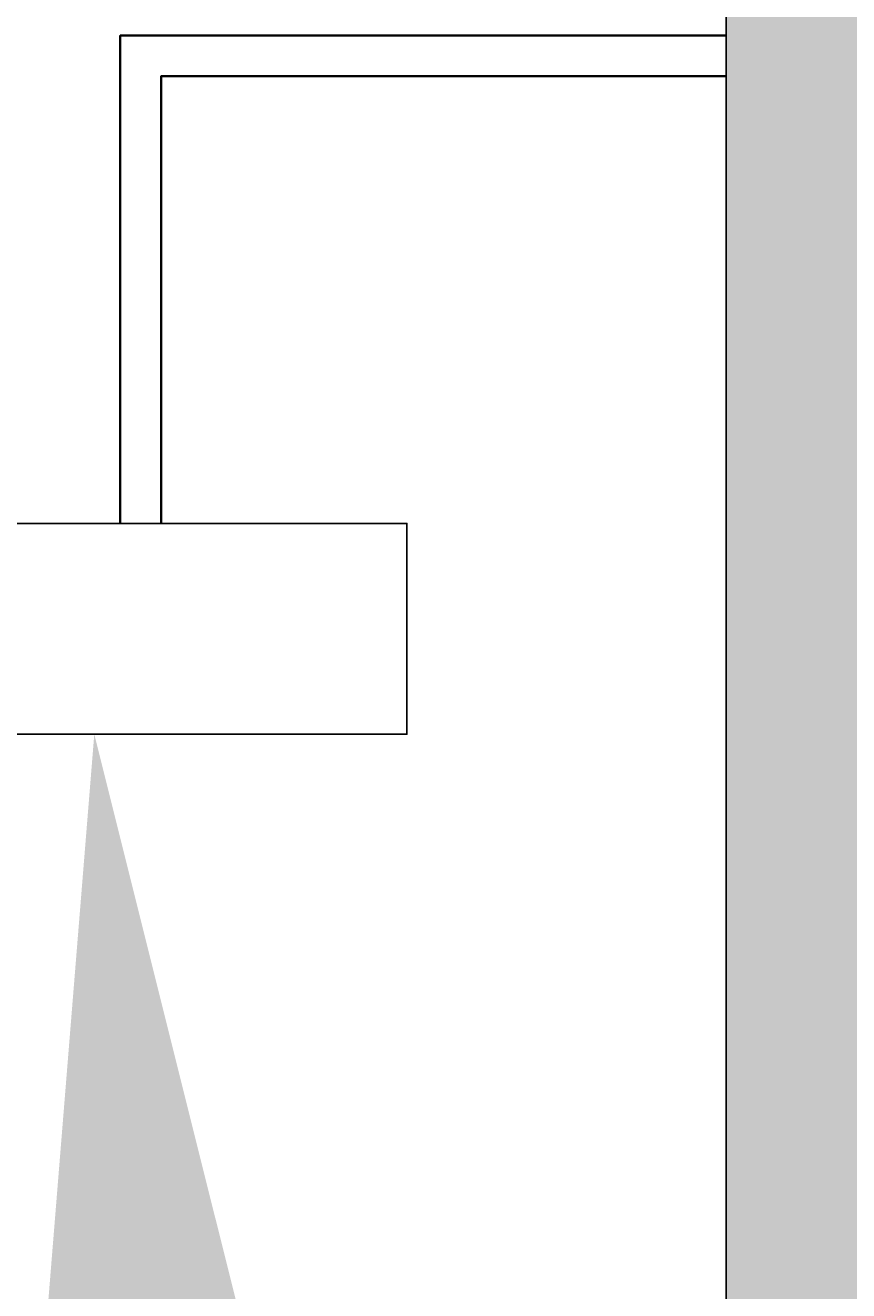
# Model space of a CAD drawing. Units: millimetres. Extents: x -22994 to 29398, y -19990 to 20176.
# Tile 15 of 135: x 79 to 99, y 21 to 52. Entities that reach past the tile are written whole.
import ezdxf
from ezdxf import colors
from ezdxf.entities.mleader import LeaderData, LeaderLine
from ezdxf.math import Vec2, Vec3

# ---------------------------------------------------------------- set-up
doc = ezdxf.new("R2010")
doc.units = ezdxf.units.MM
doc.header["$MEASUREMENT"] = 0
for name, color, linetype, lineweight in [('M-ANNO-TEXT', 7, 'Continuous', 25), ('M-DIMS', 2, 'Continuous', 18), ('M-EQPM', 7, 'Continuous', 25), ('M-EQPM-PATT', 7, 'Continuous', 18), ('M-PIPE', 7, 'Continuous', 35)]:
    doc.layers.add(name, color=color, linetype=linetype, lineweight=lineweight)
doc.styles.get("Standard").update_dxf_attribs({"font": 'arial.ttf'})
doc.dimstyles.get("Standard").update_dxf_attribs({"dimtxt": 0.18, "dimasz": 10000, "dimexe": 0.18, "dimexo": 0.0625, "dimgap": 0.09, "dimtad": 0, "dimtih": 1, "dimtoh": 1, "dimdec": 0, "dimzin": 0, "dimdsep": 46, "dimtxsty": 'Standard', "dimcen": 0.09, "dimadec": 0, "dimazin": 0, "dimtfac": 1, "dimtdec": 0, "dimtofl": 0, "dimtmove": 0, "dimatfit": 3, "dimfxl": 1, "dimtolj": 1, "dimtzin": 0, "dimlwd": 30, "dimarcsym": 0})

# ---------------------------------------------------------------- blocks, each defined once
blk = doc.blocks.new('*D2')
at = {"layer": 'Defpoints', "color": 0, "transparency": 16777216}
for p in [(6.677, 10.271), (290.852, 10.271), (290.852, -5.079)]:
    blk.add_point(p, dxfattribs=at)
at = {"layer": 'M-DIMS', "color": 0, "lineweight": -2, "transparency": 16777216}
for p, q in [((6.677, 10.209), (6.677, -5.259)), ((290.852, 10.209), (290.852, -5.259))]:
    blk.add_line(p, q, dxfattribs=at)
at = {"layer": 'M-DIMS', "color": 0, "lineweight": 30, "transparency": 16777216}
for p, q in [((-9993.323, -5.079), (-19993.323, -5.079)), ((10290.852, -5.079), (20290.852, -5.079))]:
    blk.add_line(p, q, dxfattribs=at)
at = {"layer": 'M-DIMS', "color": 0, "transparency": 16777216}
for points in [[(-9993.323, 1661.588), (-9993.323, -1671.745), (6.677, -5.079)], [(10290.852, 1661.588), (10290.852, -1671.745), (290.852, -5.079)]]:
    blk.add_solid(points, dxfattribs=at)
at = {"layer": 'M-DIMS', "color": 0, "transparency": 16777216, "insert": (148.765, -5.079), "char_height": 0.18, "attachment_point": 5}
blk.add_mtext('\\A1;284.2', dxfattribs=at)
blk = doc.blocks.new('*D3')
at = {"layer": 'Defpoints', "color": 0, "transparency": 16777216}
for p in [(110.265, 204.165), (110.265, 176.366), (95.833, 127.967)]:
    blk.add_point(p, dxfattribs=at)
at = {"layer": 'M-DIMS', "color": 0, "lineweight": 30, "transparency": 16777216}
for p, q in [((-9904.167, 204.165), (-19904.167, 204.165)), ((10110.265, 204.165), (20110.265, 204.165))]:
    blk.add_line(p, q, dxfattribs=at)
at = {"layer": 'M-DIMS', "color": 0, "lineweight": -2, "transparency": 16777216}
for p, q in [((95.833, 128.03), (95.833, 204.345)), ((110.265, 176.429), (110.265, 204.345))]:
    blk.add_line(p, q, dxfattribs=at)
at = {"layer": 'M-DIMS', "color": 0, "transparency": 16777216}
for points in [[(-9904.167, 1870.832), (-9904.167, -1462.501), (95.833, 204.165)], [(10110.265, 1870.832), (10110.265, -1462.501), (110.265, 204.165)]]:
    blk.add_solid(points, dxfattribs=at)
at = {"layer": 'M-DIMS', "color": 0, "transparency": 16777216, "insert": (103.049, 204.165), "char_height": 0.18, "attachment_point": 5}
blk.add_mtext('\\A1;14.432', dxfattribs=at)
blk = doc.blocks.new('*D4')
at = {"layer": 'Defpoints', "color": 0, "transparency": 16777216}
for p in [(116.265, 204.165), (110.265, 176.366), (116.265, 176.366)]:
    blk.add_point(p, dxfattribs=at)
at = {"layer": 'M-DIMS', "color": 0, "lineweight": 30, "transparency": 16777216}
for p, q in [((-9889.735, 204.165), (-19889.735, 204.165)), ((10116.265, 204.165), (20116.265, 204.165))]:
    blk.add_line(p, q, dxfattribs=at)
at = {"layer": 'M-DIMS', "color": 0, "lineweight": -2, "transparency": 16777216}
for p, q in [((110.265, 176.429), (110.265, 204.345)), ((116.265, 176.429), (116.265, 204.345))]:
    blk.add_line(p, q, dxfattribs=at)
at = {"layer": 'M-DIMS', "color": 0, "transparency": 16777216}
for points in [[(-9889.735, 1870.832), (-9889.735, -1462.501), (110.265, 204.165)], [(10116.265, 1870.832), (10116.265, -1462.501), (116.265, 204.165)]]:
    blk.add_solid(points, dxfattribs=at)
at = {"layer": 'M-DIMS', "color": 0, "transparency": 16777216, "insert": (113.265, 204.165), "char_height": 0.18, "attachment_point": 5}
blk.add_mtext('\\A1;6', dxfattribs=at)
blk = doc.blocks.new('*D5')
at = {"layer": 'Defpoints', "color": 0, "transparency": 16777216}
for p in [(181.265, 204.165), (116.265, 176.366), (181.265, 176.366)]:
    blk.add_point(p, dxfattribs=at)
at = {"layer": 'M-DIMS', "color": 0, "lineweight": 30, "transparency": 16777216}
for p, q in [((-9883.735, 204.165), (-19883.735, 204.165)), ((10181.265, 204.165), (20181.265, 204.165))]:
    blk.add_line(p, q, dxfattribs=at)
at = {"layer": 'M-DIMS', "color": 0, "lineweight": -2, "transparency": 16777216}
for p, q in [((116.265, 176.429), (116.265, 204.345)), ((181.265, 176.429), (181.265, 204.345))]:
    blk.add_line(p, q, dxfattribs=at)
at = {"layer": 'M-DIMS', "color": 0, "transparency": 16777216}
for points in [[(-9883.735, 1870.832), (-9883.735, -1462.501), (116.265, 204.165)], [(10181.265, 1870.832), (10181.265, -1462.501), (181.265, 204.165)]]:
    blk.add_solid(points, dxfattribs=at)
at = {"layer": 'M-DIMS', "color": 0, "transparency": 16777216, "insert": (148.765, 204.165), "char_height": 0.18, "attachment_point": 5}
blk.add_mtext('\\A1;65', dxfattribs=at)
blk = doc.blocks.new('*D6')
at = {"layer": 'Defpoints', "color": 0, "transparency": 16777216}
for p in [(187.265, 204.165), (181.265, 176.366), (187.265, 176.366)]:
    blk.add_point(p, dxfattribs=at)
at = {"layer": 'M-DIMS', "color": 0, "lineweight": 30, "transparency": 16777216}
for p, q in [((-9818.735, 204.165), (-19818.735, 204.165)), ((10187.265, 204.165), (20187.265, 204.165))]:
    blk.add_line(p, q, dxfattribs=at)
at = {"layer": 'M-DIMS', "color": 0, "lineweight": -2, "transparency": 16777216}
for p, q in [((181.265, 176.429), (181.265, 204.345)), ((187.265, 176.429), (187.265, 204.345))]:
    blk.add_line(p, q, dxfattribs=at)
at = {"layer": 'M-DIMS', "color": 0, "transparency": 16777216}
for points in [[(-9818.735, 1870.832), (-9818.735, -1462.501), (181.265, 204.165)], [(10187.265, 1870.832), (10187.265, -1462.501), (187.265, 204.165)]]:
    blk.add_solid(points, dxfattribs=at)
at = {"layer": 'M-DIMS', "color": 0, "transparency": 16777216, "insert": (184.265, 204.165), "char_height": 0.18, "attachment_point": 5}
blk.add_mtext('\\A1;6', dxfattribs=at)
blk = doc.blocks.new('*D7')
at = {"layer": 'Defpoints', "color": 0, "transparency": 16777216}
for p in [(201.697, 204.165), (187.265, 176.366), (201.697, 127.967)]:
    blk.add_point(p, dxfattribs=at)
at = {"layer": 'M-DIMS', "color": 0, "lineweight": 30, "transparency": 16777216}
for p, q in [((-9812.735, 204.165), (-19812.735, 204.165)), ((10201.697, 204.165), (20201.697, 204.165))]:
    blk.add_line(p, q, dxfattribs=at)
at = {"layer": 'M-DIMS', "color": 0, "lineweight": -2, "transparency": 16777216}
for p, q in [((187.265, 176.429), (187.265, 204.345)), ((201.697, 128.03), (201.697, 204.345))]:
    blk.add_line(p, q, dxfattribs=at)
at = {"layer": 'M-DIMS', "color": 0, "transparency": 16777216}
for points in [[(-9812.735, 1870.832), (-9812.735, -1462.501), (187.265, 204.165)], [(10201.697, 1870.832), (10201.697, -1462.501), (201.697, 204.165)]]:
    blk.add_solid(points, dxfattribs=at)
at = {"layer": 'M-DIMS', "color": 0, "transparency": 16777216, "insert": (194.481, 204.165), "char_height": 0.18, "attachment_point": 5}
blk.add_mtext('\\A1;14.432', dxfattribs=at)
blk = doc.blocks.new('*D8')
at = {"layer": 'Defpoints', "color": 0, "transparency": 16777216}
for p in [(227.648, 204.165), (227.648, 146.73), (201.697, 127.967)]:
    blk.add_point(p, dxfattribs=at)
at = {"layer": 'M-DIMS', "color": 0, "lineweight": 30, "transparency": 16777216}
for p, q in [((-9798.303, 204.165), (-19798.303, 204.165)), ((10227.648, 204.165), (20227.648, 204.165))]:
    blk.add_line(p, q, dxfattribs=at)
at = {"layer": 'M-DIMS', "color": 0, "lineweight": -2, "transparency": 16777216}
for p, q in [((201.697, 128.03), (201.697, 204.345)), ((227.648, 146.792), (227.648, 204.345))]:
    blk.add_line(p, q, dxfattribs=at)
at = {"layer": 'M-DIMS', "color": 0, "transparency": 16777216}
for points in [[(-9798.303, 1870.832), (-9798.303, -1462.501), (201.697, 204.165)], [(10227.648, 1870.832), (10227.648, -1462.501), (227.648, 204.165)]]:
    blk.add_solid(points, dxfattribs=at)
at = {"layer": 'M-DIMS', "color": 0, "transparency": 16777216, "insert": (214.673, 204.165), "char_height": 0.18, "attachment_point": 5}
blk.add_mtext('\\A1;25.95', dxfattribs=at)
blk = doc.blocks.new('*D9')
at = {"layer": 'Defpoints', "color": 0, "transparency": 16777216}
for p in [(187.265, 176.366), (306.202, 176.366), (290.852, 10.271)]:
    blk.add_point(p, dxfattribs=at)
at = {"layer": 'M-DIMS', "color": 0, "lineweight": 30, "transparency": 16777216}
for p, q in [((306.202, 10176.366), (306.202, 20176.366)), ((306.202, -9989.729), (306.202, -19989.729))]:
    blk.add_line(p, q, dxfattribs=at)
at = {"layer": 'M-DIMS', "color": 0, "lineweight": -2, "transparency": 16777216}
for p, q in [((187.327, 176.366), (306.382, 176.366)), ((290.915, 10.271), (306.382, 10.271))]:
    blk.add_line(p, q, dxfattribs=at)
at = {"layer": 'M-DIMS', "color": 0, "transparency": 16777216}
for points in [[(-1360.465, 10176.366), (1972.869, 10176.366), (306.202, 176.366)], [(-1360.465, -9989.729), (1972.869, -9989.729), (306.202, 10.271)]]:
    blk.add_solid(points, dxfattribs=at)
at = {"layer": 'M-DIMS', "color": 0, "transparency": 16777216, "insert": (306.202, 93.319), "char_height": 0.18, "attachment_point": 5}
blk.add_mtext('\\A1;166.1', dxfattribs=at)
blk = doc.blocks.new('*D10')
at = {"layer": 'Defpoints', "color": 0, "transparency": 16777216}
for p in [(125.65, 136.071), (133.346, 136.071), (133.346, -5.079)]:
    blk.add_point(p, dxfattribs=at)
at = {"layer": 'M-DIMS', "color": 0, "lineweight": -2, "transparency": 16777216}
for p, q in [((125.65, 136.009), (125.65, -5.259)), ((133.346, 136.009), (133.346, -5.259))]:
    blk.add_line(p, q, dxfattribs=at)
at = {"layer": 'M-DIMS', "color": 0, "lineweight": 30, "transparency": 16777216}
for p, q in [((-9874.35, -5.079), (-19874.35, -5.079)), ((10133.346, -5.079), (20133.346, -5.079))]:
    blk.add_line(p, q, dxfattribs=at)
at = {"layer": 'M-DIMS', "color": 0, "transparency": 16777216}
for points in [[(-9874.35, 1661.588), (-9874.35, -1671.745), (125.65, -5.079)], [(10133.346, 1661.588), (10133.346, -1671.745), (133.346, -5.079)]]:
    blk.add_solid(points, dxfattribs=at)
at = {"layer": 'M-DIMS', "color": 0, "transparency": 16777216, "insert": (129.498, -5.079), "char_height": 0.18, "attachment_point": 5}
blk.add_mtext('\\A1;7.696', dxfattribs=at)
blk = doc.blocks.new('*D11')
at = {"layer": 'Defpoints', "color": 0, "transparency": 16777216}
for p in [(133.346, 136.071), (135.65, 136.071), (135.65, -5.079)]:
    blk.add_point(p, dxfattribs=at)
at = {"layer": 'M-DIMS', "color": 0, "lineweight": -2, "transparency": 16777216}
for p, q in [((133.346, 136.009), (133.346, -5.259)), ((135.65, 136.009), (135.65, -5.259))]:
    blk.add_line(p, q, dxfattribs=at)
at = {"layer": 'M-DIMS', "color": 0, "lineweight": 30, "transparency": 16777216}
for p, q in [((-9866.654, -5.079), (-19866.654, -5.079)), ((10135.65, -5.079), (20135.65, -5.079))]:
    blk.add_line(p, q, dxfattribs=at)
at = {"layer": 'M-DIMS', "color": 0, "transparency": 16777216}
for points in [[(-9866.654, 1661.588), (-9866.654, -1671.745), (133.346, -5.079)], [(10135.65, 1661.588), (10135.65, -1671.745), (135.65, -5.079)]]:
    blk.add_solid(points, dxfattribs=at)
at = {"layer": 'M-DIMS', "color": 0, "transparency": 16777216, "insert": (134.498, -5.079), "char_height": 0.18, "attachment_point": 5}
blk.add_mtext('\\A1;2.304', dxfattribs=at)
blk = doc.blocks.new('*D12')
at = {"layer": 'Defpoints', "color": 0, "transparency": 16777216}
for p in [(135.65, 136.071), (145.65, 136.071), (145.65, -5.079)]:
    blk.add_point(p, dxfattribs=at)
at = {"layer": 'M-DIMS', "color": 0, "lineweight": -2, "transparency": 16777216}
for p, q in [((135.65, 136.009), (135.65, -5.259)), ((145.65, 136.009), (145.65, -5.259))]:
    blk.add_line(p, q, dxfattribs=at)
at = {"layer": 'M-DIMS', "color": 0, "lineweight": 30, "transparency": 16777216}
for p, q in [((-9864.35, -5.079), (-19864.35, -5.079)), ((10145.65, -5.079), (20145.65, -5.079))]:
    blk.add_line(p, q, dxfattribs=at)
at = {"layer": 'M-DIMS', "color": 0, "transparency": 16777216}
for points in [[(-9864.35, 1661.588), (-9864.35, -1671.745), (135.65, -5.079)], [(10145.65, 1661.588), (10145.65, -1671.745), (145.65, -5.079)]]:
    blk.add_solid(points, dxfattribs=at)
at = {"layer": 'M-DIMS', "color": 0, "transparency": 16777216, "insert": (140.65, -5.079), "char_height": 0.18, "attachment_point": 5}
blk.add_mtext('\\A1;10', dxfattribs=at)
blk = doc.blocks.new('*D13')
at = {"layer": 'Defpoints', "color": 0, "transparency": 16777216}
for p in [(145.65, 136.071), (155.65, 136.071), (155.65, -5.079)]:
    blk.add_point(p, dxfattribs=at)
at = {"layer": 'M-DIMS', "color": 0, "lineweight": -2, "transparency": 16777216}
for p, q in [((145.65, 136.009), (145.65, -5.259)), ((155.65, 136.009), (155.65, -5.259))]:
    blk.add_line(p, q, dxfattribs=at)
at = {"layer": 'M-DIMS', "color": 0, "lineweight": 30, "transparency": 16777216}
for p, q in [((-9854.35, -5.079), (-19854.35, -5.079)), ((10155.65, -5.079), (20155.65, -5.079))]:
    blk.add_line(p, q, dxfattribs=at)
at = {"layer": 'M-DIMS', "color": 0, "transparency": 16777216}
for points in [[(-9854.35, 1661.588), (-9854.35, -1671.745), (145.65, -5.079)], [(10155.65, 1661.588), (10155.65, -1671.745), (155.65, -5.079)]]:
    blk.add_solid(points, dxfattribs=at)
at = {"layer": 'M-DIMS', "color": 0, "transparency": 16777216, "insert": (150.65, -5.079), "char_height": 0.18, "attachment_point": 5}
blk.add_mtext('\\A1;10', dxfattribs=at)
blk = doc.blocks.new('*D14')
at = {"layer": 'Defpoints', "color": 0, "transparency": 16777216}
for p in [(155.65, 136.071), (165.65, 136.071), (165.65, -5.079)]:
    blk.add_point(p, dxfattribs=at)
at = {"layer": 'M-DIMS', "color": 0, "lineweight": -2, "transparency": 16777216}
for p, q in [((155.65, 136.009), (155.65, -5.259)), ((165.65, 136.009), (165.65, -5.259))]:
    blk.add_line(p, q, dxfattribs=at)
at = {"layer": 'M-DIMS', "color": 0, "lineweight": 30, "transparency": 16777216}
for p, q in [((-9844.35, -5.079), (-19844.35, -5.079)), ((10165.65, -5.079), (20165.65, -5.079))]:
    blk.add_line(p, q, dxfattribs=at)
at = {"layer": 'M-DIMS', "color": 0, "transparency": 16777216}
for points in [[(-9844.35, 1661.588), (-9844.35, -1671.745), (155.65, -5.079)], [(10165.65, 1661.588), (10165.65, -1671.745), (165.65, -5.079)]]:
    blk.add_solid(points, dxfattribs=at)
at = {"layer": 'M-DIMS', "color": 0, "transparency": 16777216, "insert": (160.65, -5.079), "char_height": 0.18, "attachment_point": 5}
blk.add_mtext('\\A1;10', dxfattribs=at)
blk = doc.blocks.new('*D15')
at = {"layer": 'Defpoints', "color": 0, "transparency": 16777216}
for p in [(173.346, 154.788), (173.346, 136.071), (306.202, 136.071)]:
    blk.add_point(p, dxfattribs=at)
at = {"layer": 'M-DIMS', "color": 0, "lineweight": 30, "transparency": 16777216}
for p, q in [((306.202, 10154.788), (306.202, 20154.788)), ((306.202, -9863.929), (306.202, -19863.929))]:
    blk.add_line(p, q, dxfattribs=at)
at = {"layer": 'M-DIMS', "color": 0, "lineweight": -2, "transparency": 16777216}
for p, q in [((173.408, 154.788), (306.382, 154.788)), ((173.408, 136.071), (306.382, 136.071))]:
    blk.add_line(p, q, dxfattribs=at)
at = {"layer": 'M-DIMS', "color": 0, "transparency": 16777216}
for points in [[(-1360.465, 10154.788), (1972.869, 10154.788), (306.202, 154.788)], [(-1360.465, -9863.929), (1972.869, -9863.929), (306.202, 136.071)]]:
    blk.add_solid(points, dxfattribs=at)
at = {"layer": 'M-DIMS', "color": 0, "transparency": 16777216, "insert": (306.202, 145.43), "char_height": 0.18, "attachment_point": 5}
blk.add_mtext('\\A1;18.717', dxfattribs=at)
blk = doc.blocks.new('*D16')
at = {"layer": 'Defpoints', "color": 0, "transparency": 16777216}
for p in [(120.17, 204.165), (110.466, 48.035), (120.17, 48.035)]:
    blk.add_point(p, dxfattribs=at)
at = {"layer": 'M-DIMS', "color": 0, "lineweight": 30, "transparency": 16777216}
for p, q in [((-9889.534, 204.165), (-19889.534, 204.165)), ((10120.17, 204.165), (20120.17, 204.165))]:
    blk.add_line(p, q, dxfattribs=at)
at = {"layer": 'M-DIMS', "color": 0, "lineweight": -2, "transparency": 16777216}
for p, q in [((110.466, 48.097), (110.466, 204.345)), ((120.17, 48.097), (120.17, 204.345))]:
    blk.add_line(p, q, dxfattribs=at)
at = {"layer": 'M-DIMS', "color": 0, "transparency": 16777216}
for points in [[(-9889.534, 1870.832), (-9889.534, -1462.501), (110.466, 204.165)], [(10120.17, 1870.832), (10120.17, -1462.501), (120.17, 204.165)]]:
    blk.add_solid(points, dxfattribs=at)
at = {"layer": 'M-DIMS', "color": 0, "transparency": 16777216, "insert": (115.318, 204.165), "char_height": 0.18, "attachment_point": 5}
blk.add_mtext('\\A1;9.704', dxfattribs=at)
blk = doc.blocks.new('*D17')
at = {"layer": 'Defpoints', "color": 0, "transparency": 16777216}
for p in [(126.17, 204.165), (120.17, 48.035), (126.17, 48.035)]:
    blk.add_point(p, dxfattribs=at)
at = {"layer": 'M-DIMS', "color": 0, "lineweight": 30, "transparency": 16777216}
for p, q in [((-9879.83, 204.165), (-19879.83, 204.165)), ((10126.17, 204.165), (20126.17, 204.165))]:
    blk.add_line(p, q, dxfattribs=at)
at = {"layer": 'M-DIMS', "color": 0, "lineweight": -2, "transparency": 16777216}
for p, q in [((120.17, 48.097), (120.17, 204.345)), ((126.17, 48.097), (126.17, 204.345))]:
    blk.add_line(p, q, dxfattribs=at)
at = {"layer": 'M-DIMS', "color": 0, "transparency": 16777216}
for points in [[(-9879.83, 1870.832), (-9879.83, -1462.501), (120.17, 204.165)], [(10126.17, 1870.832), (10126.17, -1462.501), (126.17, 204.165)]]:
    blk.add_solid(points, dxfattribs=at)
at = {"layer": 'M-DIMS', "color": 0, "transparency": 16777216, "insert": (123.17, 204.165), "char_height": 0.18, "attachment_point": 5}
blk.add_mtext('\\A1;6', dxfattribs=at)
blk = doc.blocks.new('*D18')
at = {"layer": 'Defpoints', "color": 0, "transparency": 16777216}
for p in [(132.17, 204.165), (126.17, 48.035), (132.17, 48.035)]:
    blk.add_point(p, dxfattribs=at)
at = {"layer": 'M-DIMS', "color": 0, "lineweight": 30, "transparency": 16777216}
for p, q in [((-9873.83, 204.165), (-19873.83, 204.165)), ((10132.17, 204.165), (20132.17, 204.165))]:
    blk.add_line(p, q, dxfattribs=at)
at = {"layer": 'M-DIMS', "color": 0, "lineweight": -2, "transparency": 16777216}
for p, q in [((126.17, 48.097), (126.17, 204.345)), ((132.17, 48.097), (132.17, 204.345))]:
    blk.add_line(p, q, dxfattribs=at)
at = {"layer": 'M-DIMS', "color": 0, "transparency": 16777216}
for points in [[(-9873.83, 1870.832), (-9873.83, -1462.501), (126.17, 204.165)], [(10132.17, 1870.832), (10132.17, -1462.501), (132.17, 204.165)]]:
    blk.add_solid(points, dxfattribs=at)
at = {"layer": 'M-DIMS', "color": 0, "transparency": 16777216, "insert": (129.17, 204.165), "char_height": 0.18, "attachment_point": 5}
blk.add_mtext('\\A1;6', dxfattribs=at)
blk = doc.blocks.new('*D19')
at = {"layer": 'Defpoints', "color": 0, "transparency": 16777216}
for p in [(138.17, 204.165), (132.17, 48.035), (138.17, 48.035)]:
    blk.add_point(p, dxfattribs=at)
at = {"layer": 'M-DIMS', "color": 0, "lineweight": 30, "transparency": 16777216}
for p, q in [((-9867.83, 204.165), (-19867.83, 204.165)), ((10138.17, 204.165), (20138.17, 204.165))]:
    blk.add_line(p, q, dxfattribs=at)
at = {"layer": 'M-DIMS', "color": 0, "lineweight": -2, "transparency": 16777216}
for p, q in [((132.17, 48.097), (132.17, 204.345)), ((138.17, 48.097), (138.17, 204.345))]:
    blk.add_line(p, q, dxfattribs=at)
at = {"layer": 'M-DIMS', "color": 0, "transparency": 16777216}
for points in [[(-9867.83, 1870.832), (-9867.83, -1462.501), (132.17, 204.165)], [(10138.17, 1870.832), (10138.17, -1462.501), (138.17, 204.165)]]:
    blk.add_solid(points, dxfattribs=at)
at = {"layer": 'M-DIMS', "color": 0, "transparency": 16777216, "insert": (135.17, 204.165), "char_height": 0.18, "attachment_point": 5}
blk.add_mtext('\\A1;6', dxfattribs=at)
blk = doc.blocks.new('*D20')
at = {"layer": 'Defpoints', "color": 0, "transparency": 16777216}
for p in [(144.17, 204.165), (138.17, 48.035), (144.17, 48.035)]:
    blk.add_point(p, dxfattribs=at)
at = {"layer": 'M-DIMS', "color": 0, "lineweight": 30, "transparency": 16777216}
for p, q in [((-9861.83, 204.165), (-19861.83, 204.165)), ((10144.17, 204.165), (20144.17, 204.165))]:
    blk.add_line(p, q, dxfattribs=at)
at = {"layer": 'M-DIMS', "color": 0, "lineweight": -2, "transparency": 16777216}
for p, q in [((138.17, 48.097), (138.17, 204.345)), ((144.17, 48.097), (144.17, 204.345))]:
    blk.add_line(p, q, dxfattribs=at)
at = {"layer": 'M-DIMS', "color": 0, "transparency": 16777216}
for points in [[(-9861.83, 1870.832), (-9861.83, -1462.501), (138.17, 204.165)], [(10144.17, 1870.832), (10144.17, -1462.501), (144.17, 204.165)]]:
    blk.add_solid(points, dxfattribs=at)
at = {"layer": 'M-DIMS', "color": 0, "transparency": 16777216, "insert": (141.17, 204.165), "char_height": 0.18, "attachment_point": 5}
blk.add_mtext('\\A1;6', dxfattribs=at)
blk = doc.blocks.new('*D21')
at = {"layer": 'Defpoints', "color": 0, "transparency": 16777216}
for p in [(149.116, 204.165), (144.17, 48.035), (149.116, 48.035)]:
    blk.add_point(p, dxfattribs=at)
at = {"layer": 'M-DIMS', "color": 0, "lineweight": 30, "transparency": 16777216}
for p, q in [((-9855.83, 204.165), (-19855.83, 204.165)), ((10149.116, 204.165), (20149.116, 204.165))]:
    blk.add_line(p, q, dxfattribs=at)
at = {"layer": 'M-DIMS', "color": 0, "lineweight": -2, "transparency": 16777216}
for p, q in [((144.17, 48.097), (144.17, 204.345)), ((149.116, 48.097), (149.116, 204.345))]:
    blk.add_line(p, q, dxfattribs=at)
at = {"layer": 'M-DIMS', "color": 0, "transparency": 16777216}
for points in [[(-9855.83, 1870.832), (-9855.83, -1462.501), (144.17, 204.165)], [(10149.116, 1870.832), (10149.116, -1462.501), (149.116, 204.165)]]:
    blk.add_solid(points, dxfattribs=at)
at = {"layer": 'M-DIMS', "color": 0, "transparency": 16777216, "insert": (146.643, 204.165), "char_height": 0.18, "attachment_point": 5}
blk.add_mtext('\\A1;4.945', dxfattribs=at)
blk = doc.blocks.new('*D22')
at = {"layer": 'Defpoints', "color": 0, "transparency": 16777216}
for p in [(149.116, 30.99), (155.116, 30.99), (155.116, -5.079)]:
    blk.add_point(p, dxfattribs=at)
at = {"layer": 'M-DIMS', "color": 0, "lineweight": -2, "transparency": 16777216}
for p, q in [((149.116, 30.927), (149.116, -5.259)), ((155.116, 30.927), (155.116, -5.259))]:
    blk.add_line(p, q, dxfattribs=at)
at = {"layer": 'M-DIMS', "color": 0, "lineweight": 30, "transparency": 16777216}
for p, q in [((-9850.884, -5.079), (-19850.884, -5.079)), ((10155.116, -5.079), (20155.116, -5.079))]:
    blk.add_line(p, q, dxfattribs=at)
at = {"layer": 'M-DIMS', "color": 0, "transparency": 16777216}
for points in [[(-9850.884, 1661.588), (-9850.884, -1671.745), (149.116, -5.079)], [(10155.116, 1661.588), (10155.116, -1671.745), (155.116, -5.079)]]:
    blk.add_solid(points, dxfattribs=at)
at = {"layer": 'M-DIMS', "color": 0, "transparency": 16777216, "insert": (152.116, -5.079), "char_height": 0.18, "attachment_point": 5}
blk.add_mtext('\\A1;6', dxfattribs=at)
blk = doc.blocks.new('*D23')
at = {"layer": 'Defpoints', "color": 0, "transparency": 16777216}
for p in [(155.116, 30.99), (161.116, 30.99), (161.116, -5.079)]:
    blk.add_point(p, dxfattribs=at)
at = {"layer": 'M-DIMS', "color": 0, "lineweight": -2, "transparency": 16777216}
for p, q in [((155.116, 30.927), (155.116, -5.259)), ((161.116, 30.927), (161.116, -5.259))]:
    blk.add_line(p, q, dxfattribs=at)
at = {"layer": 'M-DIMS', "color": 0, "lineweight": 30, "transparency": 16777216}
for p, q in [((-9844.884, -5.079), (-19844.884, -5.079)), ((10161.116, -5.079), (20161.116, -5.079))]:
    blk.add_line(p, q, dxfattribs=at)
at = {"layer": 'M-DIMS', "color": 0, "transparency": 16777216}
for points in [[(-9844.884, 1661.588), (-9844.884, -1671.745), (155.116, -5.079)], [(10161.116, 1661.588), (10161.116, -1671.745), (161.116, -5.079)]]:
    blk.add_solid(points, dxfattribs=at)
at = {"layer": 'M-DIMS', "color": 0, "transparency": 16777216, "insert": (158.116, -5.079), "char_height": 0.18, "attachment_point": 5}
blk.add_mtext('\\A1;6', dxfattribs=at)
blk = doc.blocks.new('*D24')
at = {"layer": 'Defpoints', "color": 0, "transparency": 16777216}
for p in [(161.116, 30.99), (166.439, 30.99), (166.439, -5.079)]:
    blk.add_point(p, dxfattribs=at)
at = {"layer": 'M-DIMS', "color": 0, "lineweight": -2, "transparency": 16777216}
for p, q in [((161.116, 30.927), (161.116, -5.259)), ((166.439, 30.927), (166.439, -5.259))]:
    blk.add_line(p, q, dxfattribs=at)
at = {"layer": 'M-DIMS', "color": 0, "lineweight": 30, "transparency": 16777216}
for p, q in [((-9838.884, -5.079), (-19838.884, -5.079)), ((10166.439, -5.079), (20166.439, -5.079))]:
    blk.add_line(p, q, dxfattribs=at)
at = {"layer": 'M-DIMS', "color": 0, "transparency": 16777216}
for points in [[(-9838.884, 1661.588), (-9838.884, -1671.745), (161.116, -5.079)], [(10166.439, 1661.588), (10166.439, -1671.745), (166.439, -5.079)]]:
    blk.add_solid(points, dxfattribs=at)
at = {"layer": 'M-DIMS', "color": 0, "transparency": 16777216, "insert": (163.777, -5.079), "char_height": 0.18, "attachment_point": 5}
blk.add_mtext('\\A1;5.323', dxfattribs=at)
blk = doc.blocks.new('*D25')
at = {"layer": 'Defpoints', "color": 0, "transparency": 16777216}
for p in [(166.439, 30.99), (172.439, 30.99), (172.439, -5.079)]:
    blk.add_point(p, dxfattribs=at)
at = {"layer": 'M-DIMS', "color": 0, "lineweight": -2, "transparency": 16777216}
for p, q in [((166.439, 30.927), (166.439, -5.259)), ((172.439, 30.927), (172.439, -5.259))]:
    blk.add_line(p, q, dxfattribs=at)
at = {"layer": 'M-DIMS', "color": 0, "lineweight": 30, "transparency": 16777216}
for p, q in [((-9833.561, -5.079), (-19833.561, -5.079)), ((10172.439, -5.079), (20172.439, -5.079))]:
    blk.add_line(p, q, dxfattribs=at)
at = {"layer": 'M-DIMS', "color": 0, "transparency": 16777216}
for points in [[(-9833.561, 1661.588), (-9833.561, -1671.745), (166.439, -5.079)], [(10172.439, 1661.588), (10172.439, -1671.745), (172.439, -5.079)]]:
    blk.add_solid(points, dxfattribs=at)
at = {"layer": 'M-DIMS', "color": 0, "transparency": 16777216, "insert": (169.439, -5.079), "char_height": 0.18, "attachment_point": 5}
blk.add_mtext('\\A1;6', dxfattribs=at)
blk = doc.blocks.new('*D26')
at = {"layer": 'Defpoints', "color": 0, "transparency": 16777216}
for p in [(172.439, 30.99), (178.439, 30.99), (178.439, -5.079)]:
    blk.add_point(p, dxfattribs=at)
at = {"layer": 'M-DIMS', "color": 0, "lineweight": -2, "transparency": 16777216}
for p, q in [((172.439, 30.927), (172.439, -5.259)), ((178.439, 30.927), (178.439, -5.259))]:
    blk.add_line(p, q, dxfattribs=at)
at = {"layer": 'M-DIMS', "color": 0, "lineweight": 30, "transparency": 16777216}
for p, q in [((-9827.561, -5.079), (-19827.561, -5.079)), ((10178.439, -5.079), (20178.439, -5.079))]:
    blk.add_line(p, q, dxfattribs=at)
at = {"layer": 'M-DIMS', "color": 0, "transparency": 16777216}
for points in [[(-9827.561, 1661.588), (-9827.561, -1671.745), (172.439, -5.079)], [(10178.439, 1661.588), (10178.439, -1671.745), (178.439, -5.079)]]:
    blk.add_solid(points, dxfattribs=at)
at = {"layer": 'M-DIMS', "color": 0, "transparency": 16777216, "insert": (175.439, -5.079), "char_height": 0.18, "attachment_point": 5}
blk.add_mtext('\\A1;6', dxfattribs=at)
blk = doc.blocks.new('*D27')
at = {"layer": 'Defpoints', "color": 0, "transparency": 16777216}
for p in [(178.439, 30.99), (188.117, 30.99), (188.117, -5.079)]:
    blk.add_point(p, dxfattribs=at)
at = {"layer": 'M-DIMS', "color": 0, "lineweight": -2, "transparency": 16777216}
for p, q in [((178.439, 30.927), (178.439, -5.259)), ((188.117, 30.927), (188.117, -5.259))]:
    blk.add_line(p, q, dxfattribs=at)
at = {"layer": 'M-DIMS', "color": 0, "lineweight": 30, "transparency": 16777216}
for p, q in [((-9821.561, -5.079), (-19821.561, -5.079)), ((10188.117, -5.079), (20188.117, -5.079))]:
    blk.add_line(p, q, dxfattribs=at)
at = {"layer": 'M-DIMS', "color": 0, "transparency": 16777216}
for points in [[(-9821.561, 1661.588), (-9821.561, -1671.745), (178.439, -5.079)], [(10188.117, 1661.588), (10188.117, -1671.745), (188.117, -5.079)]]:
    blk.add_solid(points, dxfattribs=at)
at = {"layer": 'M-DIMS', "color": 0, "transparency": 16777216, "insert": (183.278, -5.079), "char_height": 0.18, "attachment_point": 5}
blk.add_mtext('\\A1;9.679', dxfattribs=at)
blk = doc.blocks.new('*D28')
at = {"layer": 'Defpoints', "color": 0, "transparency": 16777216}
for p in [(188.117, 48.035), (306.202, 48.035), (188.117, 30.99)]:
    blk.add_point(p, dxfattribs=at)
at = {"layer": 'M-DIMS', "color": 0, "lineweight": 30, "transparency": 16777216}
for p, q in [((306.202, 10048.035), (306.202, 20048.035)), ((306.202, -9969.01), (306.202, -19969.01))]:
    blk.add_line(p, q, dxfattribs=at)
at = {"layer": 'M-DIMS', "color": 0, "lineweight": -2, "transparency": 16777216}
for p, q in [((188.18, 48.035), (306.382, 48.035)), ((188.18, 30.99), (306.382, 30.99))]:
    blk.add_line(p, q, dxfattribs=at)
at = {"layer": 'M-DIMS', "color": 0, "transparency": 16777216}
for points in [[(-1360.465, 10048.035), (1972.869, 10048.035), (306.202, 48.035)], [(-1360.465, -9969.01), (1972.869, -9969.01), (306.202, 30.99)]]:
    blk.add_solid(points, dxfattribs=at)
at = {"layer": 'M-DIMS', "color": 0, "transparency": 16777216, "insert": (306.202, 39.512), "char_height": 0.18, "attachment_point": 5}
blk.add_mtext('\\A1;17.045', dxfattribs=at)
blk = doc.blocks.new('*D29')
at = {"layer": 'Defpoints', "color": 0, "transparency": 16777216}
for p in [(36.801, 80.045), (64.03, 80.045)]:
    blk.add_point(p, dxfattribs=at)
at = {"layer": 'M-DIMS', "color": 0, "lineweight": -2, "transparency": 16777216}
for p, q in [((50.325, 80.045), (50.505, 80.045)), ((50.415, 79.955), (50.415, 80.135))]:
    blk.add_line(p, q, dxfattribs=at)
at = {"layer": 'M-DIMS', "color": 0, "lineweight": 30, "transparency": 16777216}
blk.add_line((20064.03, 80.03), (10064.03, 80.038), dxfattribs=at)
at = {"layer": 'M-DIMS', "color": 0, "transparency": 16777216}
blk.add_solid([(10064.031, 1746.704), (10064.028, -1586.629), (64.03, 80.045)], dxfattribs=at)
at = {"layer": 'M-DIMS', "color": 0, "transparency": 16777216, "insert": (20064.521, 80.03), "char_height": 0.18, "attachment_point": 5}
blk.add_mtext('\\A1;∅27.23', dxfattribs=at)
blk = doc.blocks.new('*D36')
at = {"layer": 'Defpoints', "color": 0, "transparency": 16777216}
for p in [(46.39, 31.303), (46.387, 26.593)]:
    blk.add_point(p, dxfattribs=at)
at = {"layer": 'M-DIMS', "color": 0, "lineweight": 30, "transparency": 16777216}
for p, q in [((57.15, 20031.301), (51.77, 10031.302)), ((10057.15, 20031.301), (57.15, 20031.301))]:
    blk.add_line(p, q, dxfattribs=at)
at = {"layer": 'M-DIMS', "color": 0, "lineweight": -2, "transparency": 16777216}
for p, q in [((46.299, 28.948), (46.479, 28.948)), ((46.389, 28.858), (46.389, 29.038))]:
    blk.add_line(p, q, dxfattribs=at)
at = {"layer": 'M-DIMS', "color": 0, "transparency": 16777216}
blk.add_solid([(-1614.896, 10032.199), (1718.436, 10030.405), (46.39, 31.303)], dxfattribs=at)
at = {"layer": 'M-DIMS', "color": 0, "transparency": 16777216, "insert": (10057.554, 20031.301), "char_height": 0.18, "attachment_point": 5}
blk.add_mtext('\\A1;∅4.71', dxfattribs=at)
blk = doc.blocks.new('*D37')
at = {"layer": 'Defpoints', "color": 0, "transparency": 16777216}
for p in [(54.834, 118.615), (59.494, 118.614)]:
    blk.add_point(p, dxfattribs=at)
at = {"layer": 'M-DIMS', "color": 0, "lineweight": -2, "transparency": 16777216}
for p, q in [((57.074, 118.614), (57.254, 118.614)), ((57.164, 118.524), (57.164, 118.704))]:
    blk.add_line(p, q, dxfattribs=at)
at = {"layer": 'M-DIMS', "color": 0, "lineweight": 30, "transparency": 16777216}
blk.add_line((20059.493, 116.253), (10059.494, 117.434), dxfattribs=at)
at = {"layer": 'M-DIMS', "color": 0, "transparency": 16777216}
blk.add_solid([(10059.69, 1784.1), (10059.297, -1549.233), (59.494, 118.614)], dxfattribs=at)
at = {"layer": 'M-DIMS', "color": 0, "transparency": 16777216, "insert": (20059.985, 116.253), "char_height": 0.18, "attachment_point": 5}
blk.add_mtext('\\A1;∅4.659', dxfattribs=at)

msp = doc.modelspace()

# ---------------------------------------------------------------- hatches: boundary and pattern name
at = {"layer": 'M-EQPM-PATT'}
h = msp.add_hatch(color=256, dxfattribs=at)
h.set_gradient(color1=(205, 32, 39), color2=(205, 32, 39), tint=1)
h.paths.add_polyline_path([(116.2647, 150.3662), (116.2647, 170.3662), (116.2647, 176.3662), (110.2647, 176.3662), (110.2647, 152.0276), (95.8327, 127.967), (95.8327, 16.6063), (201.6967, 16.6063), (201.6967, 127.967), (187.2647, 152.0276), (187.2647, 176.3662), (181.2647, 176.3662), (181.2647, 170.3662), (181.2647, 150.3662), (195.6967, 126.3055), (195.6967, 22.6063), (101.8327, 22.6063), (101.8327, 126.3055)])
h.paths.add_polyline_path([(185.2208, 88.6347), (101.8327, 88.6347), (101.8327, 87.6347), (182.8066, 87.6347), (178.7313, 83.5594), (195.6967, 83.5594), (195.6967, 84.5594), (181.1455, 84.5594)], flags=17)
h.paths.add_polyline_path([(95.8327, 88.6347), (60.9779, 88.6347, -0.0228552), (61.7178, 87.6347), (95.8327, 87.6347)])
h.paths.add_polyline_path([(215.6212, 86.5189), (215.6212, 80.5999), (220.5095, 83.5594)])
h.paths.add_polyline_path([(215.6212, 84.5594), (201.6967, 84.5594), (201.6967, 83.5594), (215.6212, 83.5594)])
h.paths.add_polyline_path([(225.3978, 86.5189), (220.5095, 83.5594), (225.3978, 80.5999)])
h.paths.add_polyline_path([(231.6256, 84.5594), (225.3978, 84.5594), (225.3978, 83.5594), (231.6256, 83.5594)])

# ---------------------------------------------------------------- linework, layer by layer
at = {"layer": 'M-EQPM'}
for points in [[(110.2647, 176.3662), (110.2647, 152.0276), (95.8327, 127.967), (95.8327, 16.6063), (201.6967, 16.6063), (201.6967, 127.967), (187.2647, 152.0276), (187.2647, 176.3662)], [(75.6375, 39.9986), (88.0111, 39.9986), (88.0111, 34.8308), (75.6375, 34.8308)]]:
    msp.add_lwpolyline(points, close=True, dxfattribs=at)
at = {"layer": 'M-PIPE'}
for points in [[(95.8327, 51.9576), (80.9868, 51.9576), (80.9868, 39.9986)], [(95.8327, 50.9576), (81.9868, 50.9576), (81.9868, 39.9986)]]:
    msp.add_lwpolyline(points, dxfattribs=at)

# ---------------------------------------------------------------- dimensions: what is measured, and where the dimension line sits
at = {"layer": 'M-DIMS'}
for base, p1, p2, override, picture, middle in [((306.202, 176.3662), (290.852, 10.2713), (187.2647, 176.3662), {"dimdec": 1, "dimlfac": 1, "dimrnd": 0, "dimzin": 0, "dimdsep": 46, "dimlunit": 2}, '*D9', (306.202, 93.3187)), ((306.202, 136.0713), (173.3459, 154.788), (173.3459, 136.0713), {"dimdec": 3, "dimlfac": 1, "dimrnd": 0, "dimzin": 0, "dimdsep": 46, "dimlunit": 2}, '*D15', (306.202, 145.4297)), ((306.202, 48.0349), (188.1175, 30.9895), (188.1175, 48.0349), {"dimdec": 3, "dimlfac": 1, "dimrnd": 0, "dimzin": 0, "dimdsep": 46, "dimlunit": 2}, '*D28', (306.202, 39.5122))]:
    dim = msp.add_linear_dim(base=base, p1=p1, p2=p2, angle=90, dimstyle='Standard', override=override, dxfattribs=at)
    dim.commit()
    dim.dimension.update_dxf_attribs({"geometry": picture, "text_midpoint": middle})
dim = msp.add_diameter_dim_2p(p1=(46.3875, 26.5934), p2=(46.39, 31.3035), dimstyle='Standard', override={"dimdec": 2, "dimlfac": 1, "dimrnd": 0, "dimzin": 0, "dimdsep": 46, "dimlunit": 2}, dxfattribs=at)
dim.commit()
dim.dimension.update_dxf_attribs({"geometry": '*D36', "text_midpoint": (10057.5542, 20031.3006), "dimtype": 163})
for base, p1, p2, override, picture, middle in [((110.2647, 204.1654), (95.8327, 127.967), (110.2647, 176.3662), {"dimdec": 3, "dimlfac": 1, "dimrnd": 0, "dimzin": 0, "dimdsep": 46, "dimlunit": 2}, '*D3', (103.0487, 204.1654)), ((116.2647, 204.1654), (110.2647, 176.3662), (116.2647, 176.3662), {"dimdec": 0, "dimlfac": 1, "dimrnd": 0, "dimzin": 0, "dimdsep": 46, "dimlunit": 2}, '*D4', (113.2647, 204.1654)), ((120.1702, 204.1654), (110.4658, 48.0349), (120.1702, 48.0349), {"dimdec": 3, "dimlfac": 1, "dimrnd": 0, "dimzin": 0, "dimdsep": 46, "dimlunit": 2}, '*D16', (115.318, 204.1654)), ((181.2647, 204.1654), (116.2647, 176.3662), (181.2647, 176.3662), {"dimdec": 0, "dimlfac": 1, "dimrnd": 0, "dimzin": 0, "dimdsep": 46, "dimlunit": 2}, '*D5', (148.7647, 204.1654)), ((126.1702, 204.1654), (120.1702, 48.0349), (126.1702, 48.0349), {"dimdec": 0, "dimlfac": 1, "dimrnd": 0, "dimzin": 0, "dimdsep": 46, "dimlunit": 2}, '*D17', (123.1702, 204.1654)), ((132.1702, 204.1654), (126.1702, 48.0349), (132.1702, 48.0349), {"dimdec": 0, "dimlfac": 1, "dimrnd": 0, "dimzin": 0, "dimdsep": 46, "dimlunit": 2}, '*D18', (129.1702, 204.1654)), ((138.1702, 204.1654), (132.1702, 48.0349), (138.1702, 48.0349), {"dimdec": 0, "dimlfac": 1, "dimrnd": 0, "dimzin": 0, "dimdsep": 46, "dimlunit": 2}, '*D19', (135.1702, 204.1654)), ((144.1702, 204.1654), (138.1702, 48.0349), (144.1702, 48.0349), {"dimdec": 0, "dimlfac": 1, "dimrnd": 0, "dimzin": 0, "dimdsep": 46, "dimlunit": 2}, '*D20', (141.1702, 204.1654)), ((149.11567, 204.16539), (144.17023, 48.03494), (149.11567, 48.03494), {"dimdec": 3, "dimlfac": 1, "dimrnd": 0, "dimzin": 0, "dimdsep": 46, "dimlunit": 2}, '*D21', (146.64295, 204.16539)), ((187.2647, 204.1654), (181.2647, 176.3662), (187.2647, 176.3662), {"dimdec": 0, "dimlfac": 1, "dimrnd": 0, "dimzin": 0, "dimdsep": 46, "dimlunit": 2}, '*D6', (184.2647, 204.1654)), ((201.6967, 204.1654), (187.2647, 176.3662), (201.6967, 127.967), {"dimdec": 3, "dimlfac": 1, "dimrnd": 0, "dimzin": 0, "dimdsep": 46, "dimlunit": 2}, '*D7', (194.4807, 204.1654)), ((227.6485, 204.1654), (201.6967, 127.967), (227.6485, 146.7296), {"dimdec": 2, "dimlfac": 1, "dimrnd": 0, "dimzin": 0, "dimdsep": 46, "dimlunit": 2}, '*D8', (214.6726, 204.1654)), ((290.852, -5.0787), (6.6773, 10.2713), (290.852, 10.2713), {"dimdec": 1, "dimlfac": 1, "dimrnd": 0, "dimzin": 0, "dimdsep": 46, "dimlunit": 2}, '*D2', (148.7647, -5.0787)), ((133.3459, -5.0787), (125.6498, 136.0713), (133.3459, 136.0713), {"dimdec": 3, "dimlfac": 1, "dimrnd": 0, "dimzin": 0, "dimdsep": 46, "dimlunit": 2}, '*D10', (129.4978, -5.0787)), ((135.6498, -5.0787), (133.3459, 136.0713), (135.6498, 136.0713), {"dimdec": 3, "dimlfac": 1, "dimrnd": 0, "dimzin": 0, "dimdsep": 46, "dimlunit": 2}, '*D11', (134.4978, -5.0787)), ((145.6498, -5.0787), (135.6498, 136.0713), (145.6498, 136.0713), {"dimdec": 0, "dimlfac": 1, "dimrnd": 0, "dimzin": 0, "dimdsep": 46, "dimlunit": 2}, '*D12', (140.6498, -5.0787)), ((155.6498, -5.0787), (145.6498, 136.0713), (155.6498, 136.0713), {"dimdec": 0, "dimlfac": 1, "dimrnd": 0, "dimzin": 0, "dimdsep": 46, "dimlunit": 2}, '*D13', (150.6498, -5.0787)), ((155.1157, -5.0787), (149.1157, 30.9895), (155.1157, 30.9895), {"dimdec": 0, "dimlfac": 1, "dimrnd": 0, "dimzin": 0, "dimdsep": 46, "dimlunit": 2}, '*D22', (152.1157, -5.0787)), ((161.1157, -5.0787), (155.1157, 30.9895), (161.1157, 30.9895), {"dimdec": 0, "dimlfac": 1, "dimrnd": 0, "dimzin": 0, "dimdsep": 46, "dimlunit": 2}, '*D23', (158.1157, -5.0787)), ((165.6498, -5.0787), (155.6498, 136.0713), (165.6498, 136.0713), {"dimdec": 0, "dimlfac": 1, "dimrnd": 0, "dimzin": 0, "dimdsep": 46, "dimlunit": 2}, '*D14', (160.6498, -5.0787)), ((166.4387, -5.0787), (161.1157, 30.9895), (166.4387, 30.9895), {"dimdec": 3, "dimlfac": 1, "dimrnd": 0, "dimzin": 0, "dimdsep": 46, "dimlunit": 2}, '*D24', (163.7772, -5.0787)), ((172.4387, -5.0787), (166.4387, 30.9895), (172.4387, 30.9895), {"dimdec": 0, "dimlfac": 1, "dimrnd": 0, "dimzin": 0, "dimdsep": 46, "dimlunit": 2}, '*D25', (169.4387, -5.0787)), ((178.4387, -5.0787), (172.4387, 30.9895), (178.4387, 30.9895), {"dimdec": 0, "dimlfac": 1, "dimrnd": 0, "dimzin": 0, "dimdsep": 46, "dimlunit": 2}, '*D26', (175.4387, -5.0787)), ((188.1175, -5.0787), (178.4387, 30.9895), (188.1175, 30.9895), {"dimdec": 3, "dimlfac": 1, "dimrnd": 0, "dimzin": 0, "dimdsep": 46, "dimlunit": 2}, '*D27', (183.2781, -5.0787))]:
    dim = msp.add_linear_dim(base=base, p1=p1, p2=p2, dimstyle='Standard', override=override, dxfattribs=at)
    dim.commit()
    dim.dimension.update_dxf_attribs({"geometry": picture, "text_midpoint": middle})
for p1, p2, override, picture, middle in [((54.8343, 118.6145), (59.4936, 118.614), {"dimdec": 3, "dimlfac": 1, "dimrnd": 0, "dimzin": 0, "dimdsep": 46, "dimlunit": 2}, '*D37', (20059.4934, 116.2531)), ((36.8006, 80.045), (64.0296, 80.045), {"dimdec": 2, "dimlfac": 1, "dimrnd": 0, "dimzin": 0, "dimdsep": 46, "dimlunit": 2}, '*D29', (20064.0296, 80.0303))]:
    dim = msp.add_diameter_dim_2p(p1=p1, p2=p2, dimstyle='Standard', override=override, dxfattribs=at)
    dim.commit()
    dim.dimension.update_dxf_attribs({"geometry": picture, "text_midpoint": middle})

# ---------------------------------------------------------------- leaders
at = {"layer": 'M-ANNO-TEXT'}
ml = msp.add_multileader_mtext('Standard', dxfattribs=at)
ml.set_content('Distributing heater', color=256)
ml.set_leader_properties()
ml.build(insert=Vec2(0, 0))
ml.multileader.update_dxf_attribs({"dogleg_length": 0.36, "arrow_head_size": 200})
ctx = ml.context
ctx.base_point, ctx.arrow_head_size, ctx.landing_gap_size, ctx.plane_origin = Vec3(86.8201, 4.9577), 200, 0.09, Vec3(80.3507, 34.8308)
notes = []
notes.append((ctx, [(1, (1, 1, 0), (82.8058, 4.9577), (1, 0), 4.0143, [(0, [(80.3507, 34.8308)], 0, [])])]))
ctx.mtext.insert, ctx.mtext.flow_direction = Vec3(86.9101, 7.5457), 5
ml = msp.add_multileader_mtext('Standard', dxfattribs=at)
ml.set_content('Circulating pump', color=256)
ml.set_leader_properties()
ml.build(insert=Vec2(0, 0))
ml.multileader.update_dxf_attribs({"dogleg_length": 0.36, "arrow_head_size": 200})
ctx = ml.context
ctx.base_point, ctx.arrow_head_size, ctx.landing_gap_size, ctx.plane_origin = Vec3(13.008, 3.5951), 200, 0.09, Vec3(56.3887, 19.3615)
ctx.text_align_type = 2
notes.append((ctx, [(1, (1, 1, 0), (63.4296, 3.5951), (-1, 0), 8.8146, [(0, [(58.1278, 30.0354)], 0, [])])]))
ctx.mtext.insert, ctx.mtext.alignment, ctx.mtext.flow_direction = Vec3(54.525, 6.1831), 3, 5
for ctx, leaders in notes:
    for number, flags, end, landing, length, lines in leaders:
        leader = LeaderData()
        leader.index, (leader.has_last_leader_line, leader.has_dogleg_vector, leader.attachment_direction) = number, flags
        leader.last_leader_point, leader.dogleg_vector, leader.dogleg_length = Vec3(end), Vec3(landing), length
        for number, points, colour, breaks in lines:
            line = LeaderLine()
            line.index, line.vertices, line.color, line.breaks = number, Vec3.list(points), colors.encode_raw_color(colour), breaks
            leader.lines.append(line)
        ctx.leaders.append(leader)

doc.saveas('drawing.dxf')
